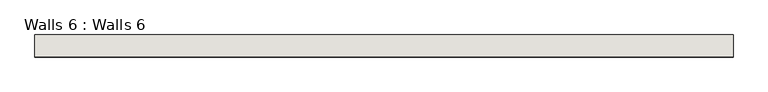
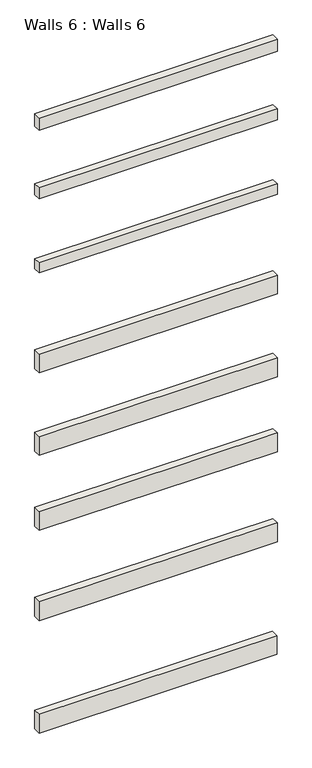
"""IFC4 building model written with IfcOpenShell, lengths in millimetres: wall geometry, Walls 6 : Walls 6."""

from ifc_helpers import new_model, si_unit, frame, origin, place, context, project, spatial, polyline, outline, extrude, source, transform, mapped, element, save


def walls_6_walls_6_eefe2e9b(model_context):
    return source(origin(), model_context, "Body", "SweptSolid", [
        extrude(outline(polyline([(-15779.6883357, -20639.6232009), (-17305.5417193, -20639.6232009), (-17305.5417193, -20591.8841974), (-15779.6883357, -20591.8841974), (-15779.6883357, -20639.6232009)])), frame((0.0, 0.0, 4689.8421352), z_axis=(0.0, 0.0, 1.0), x_axis=(1.0, 0.0, 0.0)), (0.0, 0.0, 1.0), 83.0718698),
        extrude(outline(polyline([(-15779.6883357, -20639.6232009), (-17305.5417193, -20639.6232009), (-17305.5417193, -20591.8841974), (-15779.6883357, -20591.8841974), (-15779.6883357, -20639.6232009)])), frame((0.0, 0.0, 4226.2229814), z_axis=(0.0, 0.0, 1.0), x_axis=(1.0, 0.0, 0.0)), (0.0, 0.0, 1.0), 74.7310912),
        extrude(outline(polyline([(-15779.6883357, -20639.6232009), (-17305.5417193, -20639.6232009), (-17305.5417193, -20591.8841974), (-15779.6883357, -20591.8841974), (-15779.6883357, -20639.6232009)])), frame((0.0, 0.0, 3724.7361658), z_axis=(0.0, 0.0, 1.0), x_axis=(1.0, 0.0, 0.0)), (0.0, 0.0, 1.0), 68.2179068),
        extrude(outline(polyline([(-15779.6883357, -20639.6232009), (-17305.5417193, -20639.6232009), (-17305.5417193, -20591.8841974), (-15779.6883357, -20591.8841974), (-15779.6883357, -20639.6232009)])), frame((0.0, 0.0, 3048.0), z_axis=(0.0, 0.0, 1.0), x_axis=(1.0, 0.0, 0.0)), (0.0, 0.0, 1.0), 127.0),
        extrude(outline(polyline([(-15779.6883357, -20639.6232009), (-17305.5417193, -20639.6232009), (-17305.5417193, -20591.8841974), (-15779.6883357, -20591.8841974), (-15779.6883357, -20639.6232009)])), frame((0.0, 0.0, 1981.2), z_axis=(0.0, 0.0, 1.0), x_axis=(1.0, 0.0, 0.0)), (0.0, 0.0, 1.0), 127.0),
        extrude(outline(polyline([(-15779.6883357, -20639.6232009), (-17305.5417193, -20639.6232009), (-17305.5417193, -20591.8841974), (-15779.6883357, -20591.8841974), (-15779.6883357, -20639.6232009)])), frame((0.0, 0.0, 1371.6), z_axis=(0.0, 0.0, 1.0), x_axis=(1.0, 0.0, 0.0)), (0.0, 0.0, 1.0), 127.0),
        extrude(outline(polyline([(-15781.5417193, -20639.6232009), (-17305.5417193, -20639.6232009), (-17305.5417193, -20591.8841974), (-15781.5417193, -20591.8841974), (-15781.5417193, -20639.6232009)])), frame((0.0, 0.0, 609.6), z_axis=(0.0, 0.0, 1.0), x_axis=(1.0, 0.0, 0.0)), (0.0, 0.0, 1.0), 127.0),
        extrude(outline(polyline([(-15779.6883357, -20639.6232009), (-17305.5417193, -20639.6232009), (-17305.5417193, -20591.8841974), (-15779.6883357, -20591.8841974), (-15779.6883357, -20639.6232009)])), frame((0.0, 0.0, 2489.2), z_axis=(0.0, 0.0, 1.0), x_axis=(1.0, 0.0, 0.0)), (0.0, 0.0, 1.0), 127.0),
    ])


if __name__ == "__main__":
    model = new_model("IFC4")
    model_context = context("Model", 3, world=origin())
    ifc_project = project(units=[si_unit("LENGTHUNIT", "METRE", prefix="MILLI")], contexts=[model_context])
    site = spatial("IfcSite", under=ifc_project)
    building = spatial("IfcBuilding", under=site)
    placement = place(None, origin())
    walls_6_walls_6_shape = walls_6_walls_6_eefe2e9b(model_context)
    element("IfcWall", 1, ObjectType="Walls 6 : Walls 6", at=placement, inside=building, context=model_context, shape_type="MappedRepresentation", body=[
        mapped(walls_6_walls_6_shape, transform((0.0, 0.0, 0.0), x_axis=(1.0, 0.0, 0.0), y_axis=(0.0, 1.0, 0.0), z_axis=(0.0, 0.0, 1.0))),
    ])
    save(model, "model.ifc")

# Revit data of these elements
# Element 1 (IfcWall, "Walls 6 : Walls 6")
#   Materials on its faces: "Default Wall"
# Materials
#   "Default Wall": colour RGB 80 80 80, transparency 0
